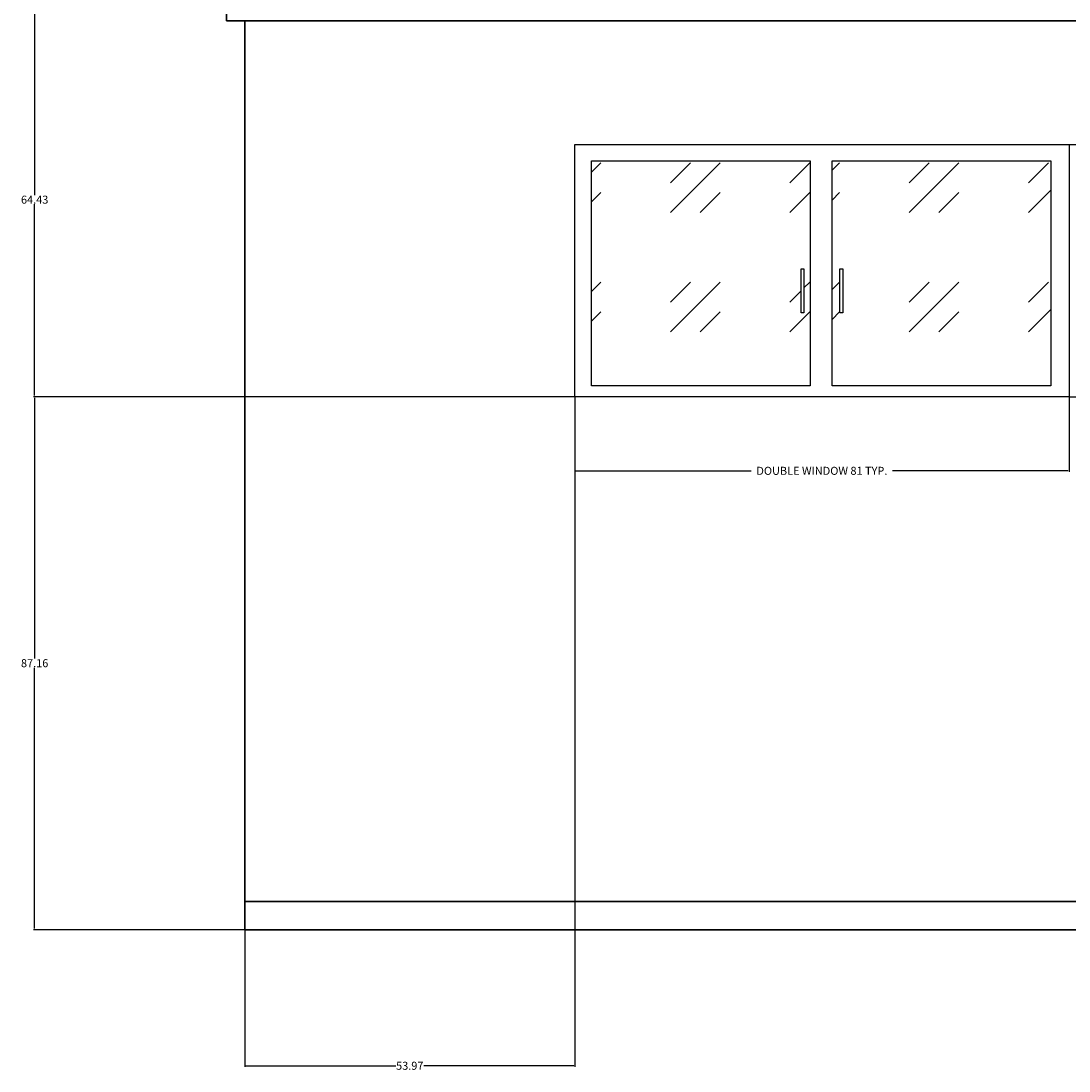
# Model space of a CAD drawing. Units: inches. Extents: x 30 to 515, y 94 to 489.
# Tile 1 of 7: x 30 to 202, y 94 to 266. Entities that reach past the tile are written whole.
import ezdxf

# ---------------------------------------------------------------- set-up
doc = ezdxf.new("R2010")
doc.units = ezdxf.units.IN
doc.header["$MEASUREMENT"] = 0
for name, color, linetype, lineweight in [('A-ANNO-DIMS', 2, 'Continuous', 18), ('A-GLAZ', 4, 'Continuous', 25), ('A-GLAZ-PATT', 8, 'Continuous', 13), ('A-WALL', 7, 'Continuous', 35)]:
    doc.layers.add(name, color=color, linetype=linetype, lineweight=lineweight)
doc.styles.get("Standard").update_dxf_attribs({"font": 'arial.ttf'})
doc.dimstyles.get("Standard").update_dxf_attribs({"dimtxt": 1.3125, "dimasz": 0.18, "dimexe": 0.18, "dimexo": 0.0625, "dimgap": 0.09, "dimtad": 0, "dimtih": 1, "dimtoh": 1, "dimdec": 4, "dimzin": 0, "dimdsep": 46, "dimlunit": 4, "dimtxsty": 'Standard', "dimcen": 0.09, "dimadec": 0, "dimazin": 0, "dimtfac": 1, "dimtdec": 4, "dimtofl": 0, "dimtmove": 0, "dimatfit": 3, "dimfxl": 1, "dimtolj": 1, "dimtzin": 0, "dimarcsym": 0})

# ---------------------------------------------------------------- blocks, each defined once
blk = doc.blocks.new('WIN-1100-DBL')
for points in [[(0, 41.22), (80.81, 41.22), (80.81, 0), (0, 0)], [(2.73, 38.58), (38.51, 38.58), (38.51, 1.75), (2.73, 1.75)], [(42.07, 38.58), (77.85, 38.58), (77.85, 1.75), (42.07, 1.75)], [(36.99, 20.89), (37.45, 20.89), (37.45, 13.69), (36.99, 13.69)], [(43.35, 20.89), (43.81, 20.89), (43.81, 13.69), (43.35, 13.69)]]:
    blk.add_lwpolyline(points, close=True)
blk = doc.blocks.new('*D2')
at = {"layer": 'A-ANNO-DIMS', "color": 0, "lineweight": -2, "transparency": 16777216}
for p, q in [((120.99, 204.03), (120.99, 191.79)), ((201.8, 204.03), (201.8, 191.79)), ((121.17, 191.97), (149.84, 191.97)), ((201.62, 191.97), (172.95, 191.97))]:
    blk.add_line(p, q, dxfattribs=at)
at = {"layer": 'A-ANNO-DIMS', "color": 0, "transparency": 16777216}
for points in [[(121.17, 192), (121.17, 191.94), (120.99, 191.97)], [(201.62, 192), (201.62, 191.94), (201.8, 191.97)]]:
    blk.add_solid(points, dxfattribs=at)
at = {"layer": 'Defpoints', "color": 0, "transparency": 16777216}
for p in [(120.99, 204.09), (201.8, 204.09), (201.8, 191.97)]:
    blk.add_point(p, dxfattribs=at)
at = {"layer": 'A-ANNO-DIMS', "color": 0, "transparency": 16777216, "insert": (161.39, 191.97), "char_height": 1.3125, "attachment_point": 5}
blk.add_mtext('\\A1;DOUBLE WINDOW 81 TYP.', dxfattribs=at)
blk = doc.blocks.new('*D3')
at = {"layer": 'A-ANNO-DIMS', "color": 0, "lineweight": -2, "transparency": 16777216}
for p, q in [((201.86, 245.32), (214.1, 245.32)), ((213.92, 245.14), (213.92, 225.45)), ((213.92, 204.27), (213.92, 223.96)), ((201.86, 204.09), (214.1, 204.09))]:
    blk.add_line(p, q, dxfattribs=at)
at = {"layer": 'A-ANNO-DIMS', "color": 0, "transparency": 16777216}
for points in [[(213.89, 245.14), (213.95, 245.14), (213.92, 245.32)], [(213.89, 204.27), (213.95, 204.27), (213.92, 204.09)]]:
    blk.add_solid(points, dxfattribs=at)
at = {"layer": 'Defpoints', "color": 0, "transparency": 16777216}
for p in [(201.8, 245.32), (213.92, 245.32), (201.8, 204.09)]:
    blk.add_point(p, dxfattribs=at)
at = {"layer": 'A-ANNO-DIMS', "color": 0, "transparency": 16777216, "insert": (213.92, 224.71), "char_height": 1.3125, "attachment_point": 5}
blk.add_mtext('\\A1;41 TYP.', dxfattribs=at)
blk = doc.blocks.new('*D7')
at = {"layer": 'A-ANNO-DIMS', "color": 0, "lineweight": -2, "transparency": 16777216}
for p, q in [((120.99, 204.03), (120.99, 94.5)), ((67.02, 121.47), (67.02, 94.5)), ((67.2, 94.68), (91.7, 94.68)), ((120.81, 94.68), (96.31, 94.68))]:
    blk.add_line(p, q, dxfattribs=at)
at = {"layer": 'A-ANNO-DIMS', "color": 0, "transparency": 16777216}
for points in [[(67.2, 94.71), (67.2, 94.65), (67.02, 94.68)], [(120.81, 94.71), (120.81, 94.65), (120.99, 94.68)]]:
    blk.add_solid(points, dxfattribs=at)
at = {"layer": 'Defpoints', "color": 0, "transparency": 16777216}
for p in [(120.99, 204.09), (67.02, 121.53), (120.99, 94.68)]:
    blk.add_point(p, dxfattribs=at)
at = {"layer": 'A-ANNO-DIMS', "color": 0, "transparency": 16777216, "insert": (94, 94.68), "char_height": 1.312, "attachment_point": 5}
blk.add_mtext('\\A1;53.97', dxfattribs=at)
blk = doc.blocks.new('*D23')
at = {"layer": 'A-ANNO-DIMS', "color": 0, "lineweight": -2, "transparency": 16777216}
for p, q in [((120.93, 204.09), (32.48, 204.09)), ((32.66, 203.91), (32.66, 161.27)), ((32.66, 117.11), (32.66, 159.75)), ((66.95, 116.93), (32.48, 116.93))]:
    blk.add_line(p, q, dxfattribs=at)
at = {"layer": 'A-ANNO-DIMS', "color": 0, "transparency": 16777216}
for points in [[(32.63, 203.91), (32.69, 203.91), (32.66, 204.09)], [(32.63, 117.11), (32.69, 117.11), (32.66, 116.93)]]:
    blk.add_solid(points, dxfattribs=at)
at = {"layer": 'Defpoints', "color": 0, "transparency": 16777216}
for p in [(32.66, 204.09), (120.99, 204.09), (67.02, 116.93)]:
    blk.add_point(p, dxfattribs=at)
at = {"layer": 'A-ANNO-DIMS', "color": 0, "transparency": 16777216, "insert": (32.66, 160.51), "char_height": 1.312, "attachment_point": 5}
blk.add_mtext('\\A1;87.16', dxfattribs=at)
blk = doc.blocks.new('*D24')
at = {"layer": 'A-ANNO-DIMS', "color": 0, "lineweight": -2, "transparency": 16777216}
for p, q in [((66.95, 268.53), (32.48, 268.53)), ((32.66, 268.35), (32.66, 237.07)), ((32.66, 204.27), (32.66, 235.55)), ((120.93, 204.09), (32.48, 204.09))]:
    blk.add_line(p, q, dxfattribs=at)
at = {"layer": 'A-ANNO-DIMS', "color": 0, "transparency": 16777216}
for points in [[(32.63, 268.35), (32.69, 268.35), (32.66, 268.53)], [(32.63, 204.27), (32.69, 204.27), (32.66, 204.09)]]:
    blk.add_solid(points, dxfattribs=at)
at = {"layer": 'Defpoints', "color": 0, "transparency": 16777216}
for p in [(32.66, 268.53), (67.02, 268.53), (120.99, 204.09)]:
    blk.add_point(p, dxfattribs=at)
at = {"layer": 'A-ANNO-DIMS', "color": 0, "transparency": 16777216, "insert": (32.66, 236.31), "char_height": 1.312, "attachment_point": 5}
blk.add_mtext('\\A1;64.43', dxfattribs=at)

msp = doc.modelspace()

# ---------------------------------------------------------------- hatches: boundary and pattern name
at = {"layer": 'A-GLAZ-PATT'}
h = msp.add_hatch(dxfattribs=at)
h.set_pattern_fill('GOST_GLASS', color=256, scale=2.3)
h.set_pattern_definition([(45, (0, 0), (19.51615, 0), [11.5, -16.1]), (45, (4.879, 0), (19.51615, 0), [4.6, -23]), (45, (0, 4.879), (19.51615, 0), [4.6, -23])])
h.paths.add_polyline_path([(141.7277, 354.4489), (122.2758, 354.4489), (122.2758, 330.4708), (141.7277, 330.4708)])
h.paths.add_polyline_path([(124.1475, 338.9533), (123.2785, 338.9533), (123.2785, 345.0981), (124.1475, 345.0981)], flags=16)
h.paths.add_polyline_path([(120.7384, 354.4489), (101.2865, 354.4489), (101.2865, 330.4708), (120.7384, 330.4708)])
h.paths.add_polyline_path([(119.0673, 338.9533), (119.0673, 345.0981), (119.9363, 345.0981), (119.9363, 338.9533)], flags=16)
h.paths.add_polyline_path([(159.5032, 242.6758), (123.7159, 242.6758), (123.7159, 205.8458), (159.5032, 205.8458)])
h.paths.add_polyline_path([(157.9822, 224.9831), (158.4447, 224.9831), (158.4447, 217.7871), (157.9822, 217.7871)], flags=16)
h.paths.add_polyline_path([(198.8424, 242.6758), (163.0551, 242.6758), (163.0551, 205.8458), (198.8424, 205.8458)])
h.paths.add_polyline_path([(164.8004, 224.9831), (164.8004, 217.7871), (164.3379, 217.7871), (164.3379, 224.9831)], flags=16)
h.paths.add_polyline_path([(389.467, 242.6758), (353.6798, 242.6758), (353.6798, 205.8458), (389.467, 205.8458)])
h.paths.add_polyline_path([(387.946, 224.9831), (388.4085, 224.9831), (388.4085, 217.7871), (387.946, 217.7871)], flags=16)
h.paths.add_polyline_path([(428.8062, 242.6758), (393.0189, 242.6758), (393.0189, 205.8458), (428.8062, 205.8458)])
h.paths.add_polyline_path([(394.7642, 224.9831), (394.7642, 217.7871), (394.3017, 217.7871), (394.3017, 224.9831)], flags=16)

# ---------------------------------------------------------------- linework, layer by layer
at = {"layer": 'A-WALL'}
for p, q in [((64.017, 268.5281), (64.017, 265.5281)), ((67.017, 265.5281), (64.017, 265.5281)), ((67.017, 121.5281), (67.017, 265.5281)), ((67.017, 265.5281), (448.0511, 265.5281)), ((67.017, 121.5281), (448.0511, 121.5281)), ((67.017, 116.9344), (67.017, 121.5281)), ((448.0511, 116.9344), (67.017, 116.9344))]:
    msp.add_line(p, q, dxfattribs=at)

# ---------------------------------------------------------------- block references
at = {"layer": 'A-GLAZ'}
msp.add_blockref('WIN-1100-DBL', (120.99, 204.094), dxfattribs=at)

# ---------------------------------------------------------------- dimensions: what is measured, and where the dimension line sits
at = {"layer": 'A-ANNO-DIMS'}
for base, p1, p2, picture, middle in [((32.6647, 268.5281), (120.9898, 204.0939), (67.017, 268.5281), '*D24', (32.6647, 236.311)), ((32.6647, 204.0939), (67.017, 116.9344), (120.9898, 204.0939), '*D23', (32.6647, 160.5141))]:
    dim = msp.add_linear_dim(base=base, p1=p1, p2=p2, angle=90, dimstyle='Standard', override={"dimdec": 2, "dimlfac": 1, "dimrnd": 0, "dimzin": 0, "dimdsep": 46, "dimlunit": 2}, dxfattribs=at)
    dim.commit()
    dim.dimension.update_dxf_attribs({"geometry": picture, "text_midpoint": middle})
dim = msp.add_linear_dim(base=(213.9186, 245.317), p1=(201.7974, 204.0939), p2=(201.7974, 245.317), angle=90, text='<> TYP.', dimstyle='Standard', override={"dimdec": 0, "dimlfac": 1, "dimrnd": 0, "dimzin": 0, "dimdsep": 46, "dimlunit": 2}, dxfattribs=at)
dim.commit()
dim.dimension.update_dxf_attribs({"geometry": '*D3', "text_midpoint": (213.9186, 224.7054)})
dim = msp.add_linear_dim(base=(120.9898, 94.6844), p1=(67.017, 121.5281), p2=(120.9898, 204.0939), dimstyle='Standard', override={"dimdec": 2, "dimlfac": 1, "dimrnd": 0, "dimzin": 0, "dimdsep": 46, "dimlunit": 2}, dxfattribs=at)
dim.commit()
dim.dimension.update_dxf_attribs({"geometry": '*D7', "text_midpoint": (94.0034, 94.6844)})
dim = msp.add_linear_dim(base=(201.7974, 191.9727), p1=(120.9898, 204.0939), p2=(201.7974, 204.0939), text='DOUBLE WINDOW <> TYP.', dimstyle='Standard', override={"dimdec": 0, "dimlfac": 1, "dimrnd": 0, "dimzin": 0, "dimdsep": 46, "dimlunit": 2}, dxfattribs=at)
dim.commit()
dim.dimension.update_dxf_attribs({"geometry": '*D2', "text_midpoint": (161.3936, 191.9727)})

doc.saveas('drawing.dxf')
